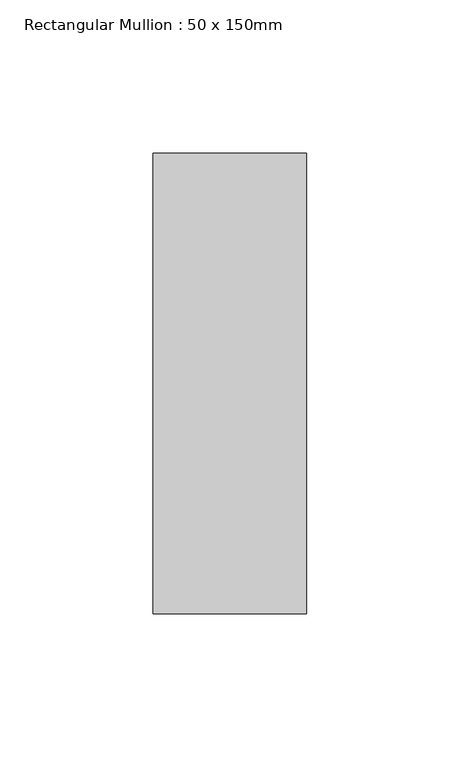
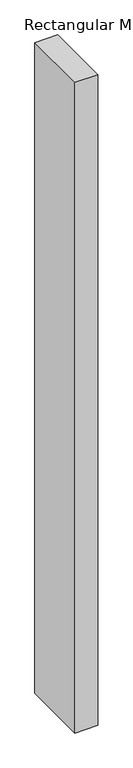
"""IFC4 building model written with IfcOpenShell, lengths in millimetres: member geometry, Rectangular Mullion : 50 x 150mm."""

from ifc_helpers import new_model, si_unit, frame, origin, place, context, project, spatial, polyline, outline, extrude, source, transform, mapped, element, save


def rectangular_mullion_50_x_150mm_63369cdd(model_context):
    return source(origin(), model_context, "Body", "SweptSolid", [
        extrude(outline(polyline([(25.0, 75.0), (25.0, -75.0), (-25.0, -75.0), (-25.0, 75.0), (25.0, 75.0)])), frame((0.0, 0.0, -1490.0), z_axis=(0.0, 0.0, 1.0), x_axis=(1.0, 0.0, 0.0)), (0.0, 0.0, 1.0), 1490.0),
    ])


if __name__ == "__main__":
    model = new_model("IFC4")
    model_context = context("Model", 3, world=origin())
    ifc_project = project(units=[si_unit("LENGTHUNIT", "METRE", prefix="MILLI")], contexts=[model_context])
    site = spatial("IfcSite", under=ifc_project)
    building = spatial("IfcBuilding", under=site)
    placement = place(None, origin())
    rectangular_mullion_50_x_150mm_shape = rectangular_mullion_50_x_150mm_63369cdd(model_context)
    element("IfcMember", 1, ObjectType="Rectangular Mullion : 50 x 150mm", at=placement, inside=building, context=model_context, shape_type="MappedRepresentation", body=[
        mapped(rectangular_mullion_50_x_150mm_shape, transform((0.0, 0.0, 0.0), x_axis=(1.0, 0.0, 0.0), y_axis=(0.0, 1.0, 0.0), z_axis=(0.0, 0.0, 1.0))),
    ])
    save(model, "model.ifc")

# Revit data of these elements
# Type "Rectangular Mullion : 50 x 150mm"
#   built-in parameter 1007304 = 0.492126 (stored number, unit not read)
#   built-in parameter 1007301 = 0.082021 (stored number, unit not read)
#   built-in parameter 1007300 = 0.082021 (stored number, unit not read)
# Element 1 (IfcMember, "Rectangular Mullion : 50 x 150mm")
#   Materials on its faces: "Aluminium"
# Materials
#   "Aluminium": class "Metal", colour RGB 247 247 247, transparency 0, Description = "Aluminium 6061", Cost = 0
